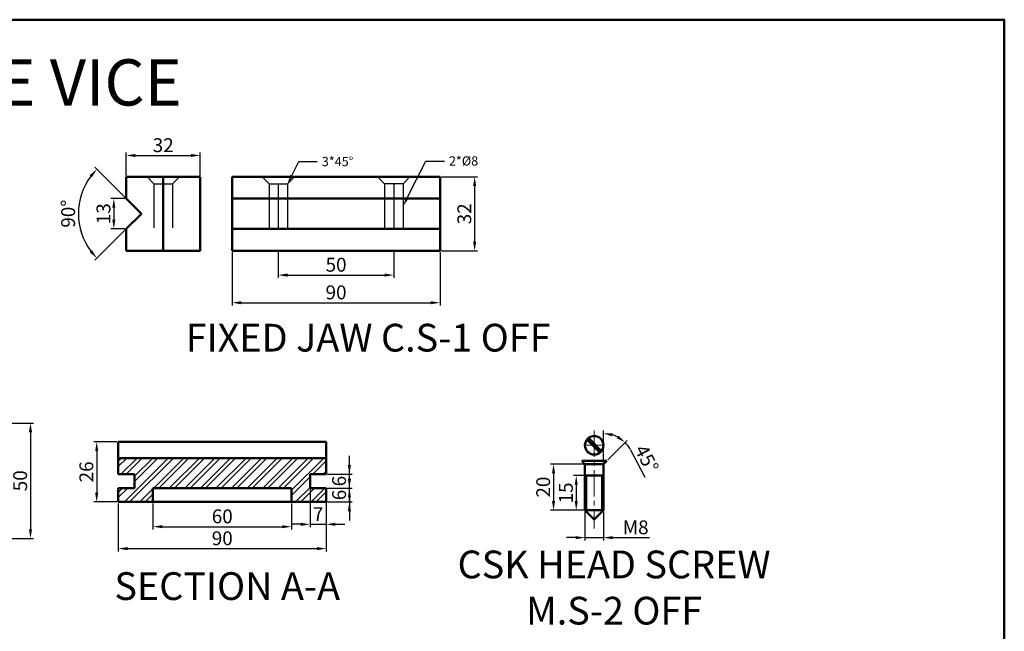
# Model space of a CAD drawing. Units: millimetres. Extents: x -1209 to -333, y 66 to 707.
# Tile 4 of 4: x -759 to -333, y 442 to 707. Entities that reach past the tile are written whole.
import ezdxf
from ezdxf import colors
from ezdxf.entities.mleader import LeaderData, LeaderLine
from ezdxf.math import Vec2, Vec3

# ---------------------------------------------------------------- set-up
doc = ezdxf.new("R2010")
doc.units = ezdxf.units.MM
doc.header["$LTSCALE"] = 1.5
doc.linetypes.add('CENTER2', pattern=[28.575, 19.05, -3.175, 3.175, -3.175])
doc.linetypes.add('DASHED', pattern=[19.05, 12.7, -6.35])
for name, color, linetype, lineweight in [('M-CNTR', 1, 'CENTER2', 18), ('M-DIMS', 2, 'Continuous', 25), ('M-HATC', 8, 'Continuous', 18), ('M-HIDN', 4, 'DASHED', 25), ('M-OUTL', 7, 'Continuous', 50), ('M-TEXT', 3, 'Continuous', 25), ('M-TTLB', 7, 'Continuous', 50)]:
    doc.layers.add(name, color=color, linetype=linetype, lineweight=lineweight)
doc.styles.get("Standard").update_dxf_attribs({"font": 'arial.ttf'})
doc.dimstyles.new('ISO-25', dxfattribs={"dimtxt": 6, "dimasz": 4, "dimexe": 1.25, "dimexo": 0.625, "dimtad": 1, "dimdec": 0, "dimtxsty": 'Standard', "dimcen": 2.5, "dimadec": 0, "dimazin": 0, "dimtfac": 1, "dimtdec": 0, "dimtmove": 0, "dimatfit": 3, "dimfxl": 1, "dimarcsym": 0})

# ---------------------------------------------------------------- blocks, each defined once
blk = doc.blocks.new('*D5')
at = {"layer": 'Defpoints', "color": 0, "transparency": 16777216}
for p in [(-788.18, 532.21), (-788.18, 482.21), (-754.08, 482.21)]:
    blk.add_point(p, dxfattribs=at)
at = {"layer": 'M-DIMS', "color": 0, "lineweight": -2, "transparency": 16777216}
for p, q in [((-787.56, 532.21), (-752.83, 532.21)), ((-754.08, 528.21), (-754.08, 486.21)), ((-787.56, 482.21), (-752.83, 482.21))]:
    blk.add_line(p, q, dxfattribs=at)
at = {"layer": 'M-DIMS', "color": 0, "transparency": 16777216}
for points in [[(-754.75, 528.21), (-753.41, 528.21), (-754.08, 532.21)], [(-754.75, 486.21), (-753.41, 486.21), (-754.08, 482.21)]]:
    blk.add_solid(points, dxfattribs=at)
at = {"layer": 'M-DIMS', "color": 0, "transparency": 16777216, "insert": (-757.77, 507.21), "char_height": 6, "attachment_point": 5, "rotation": 90}
blk.add_mtext('50', dxfattribs=at)
blk = doc.blocks.new('*D18')
at = {"layer": 'Defpoints', "color": 0, "transparency": 16777216}
for p in [(-716.06, 524.06), (-725.42, 498.06), (-716.06, 498.06)]:
    blk.add_point(p, dxfattribs=at)
at = {"layer": 'M-DIMS', "color": 0, "lineweight": -2, "transparency": 16777216}
for p, q in [((-716.69, 524.06), (-726.67, 524.06)), ((-725.42, 520.06), (-725.42, 502.06)), ((-716.69, 498.06), (-726.67, 498.06))]:
    blk.add_line(p, q, dxfattribs=at)
at = {"layer": 'M-DIMS', "color": 0, "transparency": 16777216}
for points in [[(-726.09, 520.06), (-724.76, 520.06), (-725.42, 524.06)], [(-726.09, 502.06), (-724.76, 502.06), (-725.42, 498.06)]]:
    blk.add_solid(points, dxfattribs=at)
at = {"layer": 'M-DIMS', "color": 0, "transparency": 16777216, "insert": (-729.11, 511.06), "char_height": 6, "attachment_point": 5, "rotation": 90}
blk.add_mtext('26', dxfattribs=at)
blk = doc.blocks.new('*D19')
at = {"layer": 'Defpoints', "color": 0, "transparency": 16777216}
for p in [(-716.06, 498.06), (-626.06, 498.06), (-626.06, 477.85)]:
    blk.add_point(p, dxfattribs=at)
at = {"layer": 'M-DIMS', "color": 0, "lineweight": -2, "transparency": 16777216}
for p, q in [((-716.06, 497.44), (-716.06, 476.6)), ((-626.06, 497.44), (-626.06, 476.6)), ((-712.06, 477.85), (-630.06, 477.85))]:
    blk.add_line(p, q, dxfattribs=at)
at = {"layer": 'M-DIMS', "color": 0, "transparency": 16777216}
for points in [[(-712.06, 478.52), (-712.06, 477.19), (-716.06, 477.85)], [(-630.06, 478.52), (-630.06, 477.19), (-626.06, 477.85)]]:
    blk.add_solid(points, dxfattribs=at)
at = {"layer": 'M-DIMS', "color": 0, "transparency": 16777216, "insert": (-671.06, 481.54), "char_height": 6, "attachment_point": 5}
blk.add_mtext('90', dxfattribs=at)
blk = doc.blocks.new('*D20')
at = {"layer": 'Defpoints', "color": 0, "transparency": 16777216}
for p in [(-701.06, 498.06), (-641.06, 498.06), (-641.06, 487.35)]:
    blk.add_point(p, dxfattribs=at)
at = {"layer": 'M-DIMS', "color": 0, "lineweight": -2, "transparency": 16777216}
for p, q in [((-701.06, 497.44), (-701.06, 486.1)), ((-641.06, 497.44), (-641.06, 486.1)), ((-697.06, 487.35), (-645.06, 487.35))]:
    blk.add_line(p, q, dxfattribs=at)
at = {"layer": 'M-DIMS', "color": 0, "transparency": 16777216}
for points in [[(-697.06, 488.01), (-697.06, 486.68), (-701.06, 487.35)], [(-645.06, 488.01), (-645.06, 486.68), (-641.06, 487.35)]]:
    blk.add_solid(points, dxfattribs=at)
at = {"layer": 'M-DIMS', "color": 0, "transparency": 16777216, "insert": (-671.06, 491.04), "char_height": 6, "attachment_point": 5}
blk.add_mtext('60', dxfattribs=at)
blk = doc.blocks.new('*D21')
at = {"layer": 'Defpoints', "color": 0, "transparency": 16777216}
for p in [(-633.06, 504.06), (-626.06, 504.06), (-626.06, 488.37)]:
    blk.add_point(p, dxfattribs=at)
at = {"layer": 'M-DIMS', "color": 0, "lineweight": -2, "transparency": 16777216}
for p, q in [((-633.06, 503.44), (-633.06, 487.12)), ((-626.06, 503.44), (-626.06, 487.12)), ((-637.06, 488.37), (-641.06, 488.37)), ((-633.06, 488.37), (-626.06, 488.37)), ((-622.06, 488.37), (-618.06, 488.37))]:
    blk.add_line(p, q, dxfattribs=at)
at = {"layer": 'M-DIMS', "color": 0, "transparency": 16777216}
for points in [[(-637.06, 489.04), (-637.06, 487.7), (-633.06, 488.37)], [(-622.06, 489.04), (-622.06, 487.7), (-626.06, 488.37)]]:
    blk.add_solid(points, dxfattribs=at)
at = {"layer": 'M-DIMS', "color": 0, "transparency": 16777216, "insert": (-629.56, 491.99), "char_height": 6, "attachment_point": 5}
blk.add_mtext('7', dxfattribs=at)
blk = doc.blocks.new('*D22')
at = {"layer": 'Defpoints', "color": 0, "transparency": 16777216}
for p in [(-626.06, 504.06), (-616.02, 504.06), (-626.06, 498.06)]:
    blk.add_point(p, dxfattribs=at)
at = {"layer": 'M-DIMS', "color": 0, "lineweight": -2, "transparency": 16777216}
for p, q in [((-616.02, 508.06), (-616.02, 512.06)), ((-625.44, 504.06), (-614.77, 504.06)), ((-616.02, 498.06), (-616.02, 504.06)), ((-625.44, 498.06), (-614.77, 498.06)), ((-616.02, 494.06), (-616.02, 490.06))]:
    blk.add_line(p, q, dxfattribs=at)
at = {"layer": 'M-DIMS', "color": 0, "transparency": 16777216}
for points in [[(-616.69, 508.06), (-615.35, 508.06), (-616.02, 504.06)], [(-616.69, 494.06), (-615.35, 494.06), (-616.02, 498.06)]]:
    blk.add_solid(points, dxfattribs=at)
at = {"layer": 'M-DIMS', "color": 0, "transparency": 16777216, "insert": (-619.71, 501.06), "char_height": 6, "attachment_point": 5, "rotation": 90}
blk.add_mtext('6', dxfattribs=at)
blk = doc.blocks.new('*D23')
at = {"layer": 'Defpoints', "color": 0, "transparency": 16777216}
for p in [(-626.06, 510.06), (-616.02, 510.06), (-626.06, 504.06)]:
    blk.add_point(p, dxfattribs=at)
at = {"layer": 'M-DIMS', "color": 0, "lineweight": -2, "transparency": 16777216}
for p, q in [((-616.02, 514.06), (-616.02, 518.06)), ((-625.44, 510.06), (-614.77, 510.06)), ((-616.02, 504.06), (-616.02, 510.06)), ((-625.44, 504.06), (-614.77, 504.06)), ((-616.02, 500.06), (-616.02, 496.06))]:
    blk.add_line(p, q, dxfattribs=at)
at = {"layer": 'M-DIMS', "color": 0, "transparency": 16777216}
for points in [[(-616.69, 514.06), (-615.35, 514.06), (-616.02, 510.06)], [(-616.69, 500.06), (-615.35, 500.06), (-616.02, 504.06)]]:
    blk.add_solid(points, dxfattribs=at)
at = {"layer": 'M-DIMS', "color": 0, "transparency": 16777216, "insert": (-619.71, 507.06), "char_height": 6, "attachment_point": 5, "rotation": 90}
blk.add_mtext('6', dxfattribs=at)
blk = doc.blocks.new('*D53')
at = {"layer": 'Defpoints', "color": 0, "ltscale": 0.4, "transparency": 16777216}
for p in [(-646.8, 606.73), (-596.8, 606.73), (-596.8, 596.22)]:
    blk.add_point(p, dxfattribs=at)
at = {"layer": 'M-DIMS', "color": 0, "lineweight": -2, "ltscale": 0.4, "transparency": 16777216}
for p, q in [((-646.8, 606.1), (-646.8, 594.97)), ((-596.8, 606.1), (-596.8, 594.97)), ((-642.8, 596.22), (-600.8, 596.22))]:
    blk.add_line(p, q, dxfattribs=at)
at = {"layer": 'M-DIMS', "color": 0, "ltscale": 0.4, "transparency": 16777216}
for points in [[(-642.8, 596.89), (-642.8, 595.55), (-646.8, 596.22)], [(-600.8, 596.89), (-600.8, 595.55), (-596.8, 596.22)]]:
    blk.add_solid(points, dxfattribs=at)
at = {"layer": 'M-DIMS', "color": 0, "ltscale": 0.4, "transparency": 16777216, "insert": (-621.8, 599.91), "char_height": 6, "attachment_point": 5}
blk.add_mtext('50', dxfattribs=at)
blk = doc.blocks.new('*D54')
at = {"layer": 'Defpoints', "color": 0, "ltscale": 0.4, "transparency": 16777216}
for p in [(-666.8, 606.73), (-576.8, 606.73), (-576.8, 584.26)]:
    blk.add_point(p, dxfattribs=at)
at = {"layer": 'M-DIMS', "color": 0, "lineweight": -2, "ltscale": 0.4, "transparency": 16777216}
for p, q in [((-666.8, 606.1), (-666.8, 583.01)), ((-576.8, 606.1), (-576.8, 583.01)), ((-662.8, 584.26), (-580.8, 584.26))]:
    blk.add_line(p, q, dxfattribs=at)
at = {"layer": 'M-DIMS', "color": 0, "ltscale": 0.4, "transparency": 16777216}
for points in [[(-662.8, 584.92), (-662.8, 583.59), (-666.8, 584.26)], [(-580.8, 584.92), (-580.8, 583.59), (-576.8, 584.26)]]:
    blk.add_solid(points, dxfattribs=at)
at = {"layer": 'M-DIMS', "color": 0, "ltscale": 0.4, "transparency": 16777216, "insert": (-621.8, 587.95), "char_height": 6, "attachment_point": 5}
blk.add_mtext('90', dxfattribs=at)
blk = doc.blocks.new('*D55')
at = {"layer": 'Defpoints', "color": 0, "ltscale": 0.4, "transparency": 16777216}
for p in [(-576.8, 638.73), (-576.8, 606.73), (-561.82, 606.73)]:
    blk.add_point(p, dxfattribs=at)
at = {"layer": 'M-DIMS', "color": 0, "lineweight": -2, "ltscale": 0.4, "transparency": 16777216}
for p, q in [((-576.17, 638.73), (-560.57, 638.73)), ((-561.82, 634.73), (-561.82, 610.73)), ((-576.17, 606.73), (-560.57, 606.73))]:
    blk.add_line(p, q, dxfattribs=at)
at = {"layer": 'M-DIMS', "color": 0, "ltscale": 0.4, "transparency": 16777216}
for points in [[(-562.49, 634.73), (-561.15, 634.73), (-561.82, 638.73)], [(-562.49, 610.73), (-561.15, 610.73), (-561.82, 606.73)]]:
    blk.add_solid(points, dxfattribs=at)
at = {"layer": 'M-DIMS', "color": 0, "ltscale": 0.4, "transparency": 16777216, "insert": (-565.51, 622.73), "char_height": 6, "attachment_point": 5, "rotation": 90}
blk.add_mtext('32', dxfattribs=at)
blk = doc.blocks.new('*D56')
at = {"layer": 'Defpoints', "color": 0, "ltscale": 0.4, "transparency": 16777216}
for p in [(-680.62, 647.97), (-712.62, 638.73), (-680.62, 638.73)]:
    blk.add_point(p, dxfattribs=at)
at = {"layer": 'M-DIMS', "color": 0, "lineweight": -2, "ltscale": 0.4, "transparency": 16777216}
for p, q in [((-712.62, 639.35), (-712.62, 649.22)), ((-708.62, 647.97), (-684.62, 647.97)), ((-680.62, 639.35), (-680.62, 649.22))]:
    blk.add_line(p, q, dxfattribs=at)
at = {"layer": 'M-DIMS', "color": 0, "ltscale": 0.4, "transparency": 16777216}
for points in [[(-708.62, 648.64), (-708.62, 647.31), (-712.62, 647.97)], [(-684.62, 648.64), (-684.62, 647.31), (-680.62, 647.97)]]:
    blk.add_solid(points, dxfattribs=at)
at = {"layer": 'M-DIMS', "color": 0, "ltscale": 0.4, "transparency": 16777216, "insert": (-696.62, 651.66), "char_height": 6, "attachment_point": 5}
blk.add_mtext('32', dxfattribs=at)
blk = doc.blocks.new('*D57')
at = {"layer": 'Defpoints', "color": 0, "ltscale": 0.4, "transparency": 16777216}
for p in [(-712.62, 629.33), (-718.01, 616.23), (-712.62, 616.23)]:
    blk.add_point(p, dxfattribs=at)
at = {"layer": 'M-DIMS', "color": 0, "lineweight": -2, "ltscale": 0.4, "transparency": 16777216}
for p, q in [((-713.24, 629.33), (-719.26, 629.33)), ((-718.01, 625.33), (-718.01, 620.23)), ((-713.24, 616.23), (-719.26, 616.23))]:
    blk.add_line(p, q, dxfattribs=at)
at = {"layer": 'M-DIMS', "color": 0, "ltscale": 0.4, "transparency": 16777216}
for points in [[(-718.67, 625.33), (-717.34, 625.33), (-718.01, 629.33)], [(-718.67, 620.23), (-717.34, 620.23), (-718.01, 616.23)]]:
    blk.add_solid(points, dxfattribs=at)
at = {"layer": 'M-DIMS', "color": 0, "ltscale": 0.4, "transparency": 16777216, "insert": (-721.7, 622.78), "char_height": 6, "attachment_point": 5, "rotation": 90}
blk.add_mtext('13', dxfattribs=at)
blk = doc.blocks.new('*D58')
at = {"layer": 'Defpoints', "color": 0, "ltscale": 0.4, "transparency": 16777216}
for p in [(-732.39, 629.83), (-712.62, 629.33), (-706.07, 622.78), (-706.07, 622.78), (-712.62, 616.23)]:
    blk.add_point(p, dxfattribs=at)
at = {"layer": 'M-DIMS', "color": 0, "lineweight": -2, "ltscale": 0.4, "transparency": 16777216}
for p, q in [((-713.06, 629.77), (-726.22, 642.93)), ((-713.06, 615.79), (-726.22, 602.63))]:
    blk.add_line(p, q, dxfattribs=at)
blk.add_arc((-706.07, 622.78), 27.25, 143.4187, 216.5813, dxfattribs=at)
at = {"layer": 'M-DIMS', "color": 0, "ltscale": 0.4, "transparency": 16777216}
for points in [[(-728.45, 639.45), (-727.44, 638.58), (-725.33, 642.05)], [(-727.44, 606.98), (-728.45, 606.1), (-725.33, 603.51)]]:
    blk.add_solid(points, dxfattribs=at)
at = {"layer": 'M-DIMS', "color": 0, "ltscale": 0.4, "transparency": 16777216, "insert": (-737, 622.78), "char_height": 6, "attachment_point": 5, "rotation": 90}
blk.add_mtext('90°', dxfattribs=at)
blk = doc.blocks.new('*D59')
at = {"layer": 'Defpoints', "color": 0, "ltscale": 0.4, "transparency": 16777216}
for p in [(-502.64, 527.23), (-504.65, 515.88), (-506.06, 514.46), (-506.06, 514.46), (-506.06, 494.46)]:
    blk.add_point(p, dxfattribs=at)
at = {"layer": 'M-DIMS', "color": 0, "lineweight": -2, "ltscale": 0.4, "transparency": 16777216}
for p, q in [((-506.06, 515.09), (-506.06, 528.94)), ((-504.2, 516.32), (-495.83, 524.7)), ((-494.34, 520.59), (-488.2, 508.84))]:
    blk.add_line(p, q, dxfattribs=at)
for start, end in [(62.398, 72.602), (27.602, 45)]:
    blk.add_arc((-506.06, 514.46), 13.22, start, end, dxfattribs=at)
at = {"layer": 'M-DIMS', "color": 0, "ltscale": 0.4, "transparency": 16777216}
for points in [[(-502.21, 526.42), (-502.01, 527.74), (-506.06, 527.69)], [(-499.54, 526.72), (-500.33, 525.64), (-496.71, 523.81)]]:
    blk.add_solid(points, dxfattribs=at)
at = {"layer": 'M-DIMS', "color": 0, "ltscale": 0.4, "transparency": 16777216, "insert": (-488.01, 516.42), "char_height": 6, "attachment_point": 5, "rotation": 297.602}
blk.add_mtext('45°', dxfattribs=at)
blk = doc.blocks.new('*D60')
at = {"layer": 'Defpoints', "color": 0, "ltscale": 0.4, "transparency": 16777216}
for p in [(-514.06, 514.46), (-527.66, 494.46), (-514.06, 494.46)]:
    blk.add_point(p, dxfattribs=at)
at = {"layer": 'M-DIMS', "color": 0, "lineweight": -2, "ltscale": 0.4, "transparency": 16777216}
for p, q in [((-514.69, 514.46), (-528.91, 514.46)), ((-527.66, 510.46), (-527.66, 498.46)), ((-514.69, 494.46), (-528.91, 494.46))]:
    blk.add_line(p, q, dxfattribs=at)
at = {"layer": 'M-DIMS', "color": 0, "ltscale": 0.4, "transparency": 16777216}
for points in [[(-528.33, 510.46), (-526.99, 510.46), (-527.66, 514.46)], [(-528.33, 498.46), (-526.99, 498.46), (-527.66, 494.46)]]:
    blk.add_solid(points, dxfattribs=at)
at = {"layer": 'M-DIMS', "color": 0, "ltscale": 0.4, "transparency": 16777216, "insert": (-531.35, 504.46), "char_height": 6, "attachment_point": 5, "rotation": 90}
blk.add_mtext('20', dxfattribs=at)
blk = doc.blocks.new('*D61')
at = {"layer": 'Defpoints', "color": 0, "ltscale": 0.4, "transparency": 16777216}
for p in [(-514.06, 509.46), (-517.84, 494.46), (-514.06, 494.46)]:
    blk.add_point(p, dxfattribs=at)
at = {"layer": 'M-DIMS', "color": 0, "lineweight": -2, "ltscale": 0.4, "transparency": 16777216}
for p, q in [((-514.69, 509.46), (-519.09, 509.46)), ((-517.84, 505.46), (-517.84, 498.46)), ((-514.69, 494.46), (-519.09, 494.46))]:
    blk.add_line(p, q, dxfattribs=at)
at = {"layer": 'M-DIMS', "color": 0, "ltscale": 0.4, "transparency": 16777216}
for points in [[(-518.5, 505.46), (-517.17, 505.46), (-517.84, 509.46)], [(-518.5, 498.46), (-517.17, 498.46), (-517.84, 494.46)]]:
    blk.add_solid(points, dxfattribs=at)
at = {"layer": 'M-DIMS', "color": 0, "ltscale": 0.4, "transparency": 16777216, "insert": (-521.53, 501.96), "char_height": 6, "attachment_point": 5, "rotation": 90}
blk.add_mtext('15', dxfattribs=at)
blk = doc.blocks.new('*D62')
at = {"layer": 'Defpoints', "color": 0, "ltscale": 0.4, "transparency": 16777216}
for p in [(-514.06, 494.46), (-506.06, 494.46), (-506.06, 482.61)]:
    blk.add_point(p, dxfattribs=at)
at = {"layer": 'M-DIMS', "color": 0, "lineweight": -2, "ltscale": 0.4, "transparency": 16777216}
for p, q in [((-514.06, 493.84), (-514.06, 481.36)), ((-506.06, 493.84), (-506.06, 481.36)), ((-518.06, 482.61), (-522.06, 482.61)), ((-514.06, 482.61), (-506.06, 482.61)), ((-502.06, 482.61), (-486.16, 482.61))]:
    blk.add_line(p, q, dxfattribs=at)
at = {"layer": 'M-DIMS', "color": 0, "ltscale": 0.4, "transparency": 16777216}
for points in [[(-518.06, 483.27), (-518.06, 481.94), (-514.06, 482.61)], [(-502.06, 483.27), (-502.06, 481.94), (-506.06, 482.61)]]:
    blk.add_solid(points, dxfattribs=at)
at = {"layer": 'M-DIMS', "color": 0, "ltscale": 0.4, "transparency": 16777216, "insert": (-492.11, 486.3), "char_height": 6, "attachment_point": 5}
blk.add_mtext('M8', dxfattribs=at)

msp = doc.modelspace()

# ---------------------------------------------------------------- hatches: boundary and pattern name
at = {"layer": 'M-HATC'}
h = msp.add_hatch(dxfattribs=at)
h.set_pattern_fill('ANSI32', color=256, scale=0.5)
h.set_pattern_definition([(45, (-2142.44, -526.8178), (-3.367596, 3.367596), []), (45, (-2140.195, -526.8178), (-3.367596, 3.367596), [])])
h.paths.add_polyline_path([(-641.06, 504.06), (-641.06, 498.06), (-626.06, 498.06), (-626.06, 504.06), (-633.06, 504.06), (-633.06, 510.06), (-626.06, 510.06), (-626.06, 517.06), (-638.06, 517.06), (-716.06, 517.06), (-716.06, 510.06), (-709.06, 510.06), (-709.06, 504.06), (-716.06, 504.06), (-716.06, 498.06), (-701.06, 498.06), (-701.06, 504.06)])

# ---------------------------------------------------------------- linework, layer by layer
at = {"layer": 'M-CNTR', "ltscale": 0.4}
for p, q in [((-510.06, 528.96), (-510.06, 486.51)), ((-514.06, 522.56), (-506.06, 522.56))]:
    msp.add_line(p, q, dxfattribs=at)
at = {"layer": 'M-HIDN'}
for p, q in [((-700.62, 635.73), (-703.62, 638.73)), ((-700.62, 635.73), (-700.62, 606.73)), ((-700.62, 635.73), (-692.62, 635.73)), ((-696.62, 635.73), (-696.62, 606.73)), ((-692.62, 635.73), (-689.62, 638.73)), ((-692.62, 635.73), (-692.62, 606.73)), ((-650.8, 635.73), (-653.8, 638.73)), ((-650.8, 635.73), (-650.8, 606.73)), ((-650.8, 635.73), (-642.8, 635.73)), ((-646.8, 635.73), (-646.8, 606.73)), ((-642.8, 635.73), (-639.8, 638.73)), ((-642.8, 635.73), (-642.8, 606.73)), ((-600.8, 635.73), (-603.8, 638.73)), ((-600.8, 635.73), (-600.8, 606.73)), ((-592.8, 635.73), (-600.8, 635.73)), ((-596.8, 635.73), (-596.8, 606.73)), ((-592.8, 635.73), (-589.8, 638.73)), ((-592.8, 635.73), (-592.8, 606.73))]:
    msp.add_line(p, q, dxfattribs=at)
at = {"layer": 'M-OUTL'}
for p, q in [((-712.62, 638.73), (-680.62, 638.73)), ((-712.62, 629.33), (-712.62, 638.73)), ((-700.62, 638.73), (-692.62, 638.73)), ((-680.62, 638.73), (-680.62, 606.73)), ((-576.8, 638.73), (-666.8, 638.73)), ((-666.8, 638.73), (-666.8, 606.73)), ((-592.8, 638.73), (-600.8, 638.73)), ((-576.8, 606.73), (-576.8, 638.73)), ((-666.8, 629.33), (-576.8, 629.33)), ((-712.62, 606.73), (-712.62, 616.23)), ((-666.8, 616.23), (-576.8, 616.23)), ((-680.62, 606.73), (-712.62, 606.73)), ((-666.8, 606.73), (-576.8, 606.73)), ((-716.06, 524.06), (-626.06, 524.06)), ((-716.06, 510.06), (-716.06, 524.06)), ((-626.06, 524.06), (-626.06, 510.06)), ((-638.06, 517.06), (-716.06, 517.06)), ((-626.06, 517.06), (-638.06, 517.06)), ((-709.06, 510.06), (-716.06, 510.06)), ((-709.06, 504.06), (-709.06, 510.06)), ((-626.06, 510.06), (-633.06, 510.06)), ((-633.06, 510.06), (-633.06, 504.06)), ((-716.06, 498.06), (-716.06, 504.06)), ((-709.06, 504.06), (-716.06, 504.06)), ((-641.06, 504.06), (-701.06, 504.06)), ((-701.06, 498.06), (-701.06, 504.06)), ((-641.06, 498.06), (-641.06, 504.06)), ((-626.06, 504.06), (-633.06, 504.06)), ((-626.06, 504.06), (-626.06, 498.06)), ((-626.06, 498.06), (-716.06, 498.06))]:
    msp.add_line(p, q, dxfattribs=at)
at = {"layer": 'M-OUTL', "ltscale": 0.4}
for p, q in [((-696.62, 638.73), (-696.62, 606.73)), ((-712.62, 629.33), (-706.07, 622.78)), ((-712.62, 616.23), (-706.07, 622.78)), ((-507.59, 519.38), (-513.24, 525.04)), ((-507.23, 519.74), (-512.89, 525.39)), ((-506.88, 520.09), (-512.54, 525.75)), ((-514.06, 514.46), (-515.47, 515.88)), ((-515.47, 515.88), (-504.65, 515.88)), ((-506.06, 514.46), (-504.65, 515.88)), ((-514.06, 514.46), (-506.06, 514.46)), ((-514.06, 494.46), (-514.06, 514.46)), ((-506.06, 514.46), (-506.06, 494.46)), ((-506.06, 509.46), (-514.06, 509.46)), ((-513.56, 494.46), (-513.56, 509.46)), ((-506.56, 509.46), (-506.56, 494.46)), ((-506.06, 494.46), (-514.06, 494.46)), ((-514.06, 494.46), (-510.06, 490.46)), ((-506.06, 494.46), (-510.06, 490.46))]:
    msp.add_line(p, q, dxfattribs=at)
msp.add_circle((-510.06, 522.56), 4, dxfattribs=at)
at = {"layer": 'M-TTLB', "ltscale": 0.4}
msp.add_lwpolyline([(-1209.09, 706.73), (-332.54, 706.73), (-332.54, 66.01), (-1209.09, 66.01)], close=True, dxfattribs=at)

# ---------------------------------------------------------------- texts
at = {"layer": 'M-TEXT', "ltscale": 0.4, "attachment_point": 1}
for s, width, insert, char_height in [('\\pxqc;MACHINE VICE', 213.0298, (-886.63, 689.59), 20), ('\\pxqc;FIXED JAW C.S-1 OFF', 177.8457, (-696.84, 575.13), 12), ('\\pxqc;CSK HEAD SCREW M.S-2 OFF', 177.8457, (-590.37, 477.01), 12), ('\\pxqc;SECTION A-A', 177.8457, (-757.83, 467.64), 12)]:
    msp.add_mtext_dynamic_manual_height_columns(s, width=width, gutter_width=12.5, heights=[0], dxfattribs=dict(at, insert=insert, char_height=char_height))

# ---------------------------------------------------------------- dimensions: what is measured, and where the dimension line sits
at = {"layer": 'M-DIMS', "ltscale": 0.4}
for base, p1, p2, picture, middle in [((-680.62, 647.97), (-712.62, 638.73), (-680.62, 638.73), '*D56', (-696.62, 651.66)), ((-576.8, 584.26), (-666.8, 606.73), (-576.8, 606.73), '*D54', (-621.8, 587.95)), ((-596.8, 596.22), (-646.8, 606.73), (-596.8, 606.73), '*D53', (-621.8, 599.91))]:
    dim = msp.add_linear_dim(base=base, p1=p1, p2=p2, dimstyle='ISO-25', override={"dimclrd": 0, "dimclre": 0, "dimclrt": 0}, dxfattribs=at)
    dim.commit()
    dim.dimension.update_dxf_attribs({"geometry": picture, "text_midpoint": middle})
for base, line1, line2, picture, middle in [((-732.39, 629.83), ((-712.62, 616.23), (-706.07, 622.78)), ((-712.62, 629.33), (-706.07, 622.78)), '*D58', (-737, 622.78)), ((-502.64, 527.23), ((-506.06, 514.46), (-506.06, 494.46)), ((-506.06, 514.46), (-504.65, 515.88)), '*D59', (-488.01, 516.42))]:
    dim = msp.add_angular_dim_2l(base=base, line1=line1, line2=line2, dimstyle='ISO-25', override={"dimclrd": 0, "dimclre": 0, "dimclrt": 0}, dxfattribs=at)
    dim.commit()
    dim.dimension.update_dxf_attribs({"geometry": picture, "text_midpoint": middle})
for base, p1, p2, picture, middle in [((-561.82, 606.73), (-576.8, 638.73), (-576.8, 606.73), '*D55', (-565.51, 622.73)), ((-718.01, 616.23), (-712.62, 629.33), (-712.62, 616.23), '*D57', (-721.7, 622.78)), ((-527.66, 494.46), (-514.06, 514.46), (-514.06, 494.46), '*D60', (-531.35, 504.46)), ((-517.84, 494.46), (-514.06, 509.46), (-514.06, 494.46), '*D61', (-521.53, 501.96))]:
    dim = msp.add_linear_dim(base=base, p1=p1, p2=p2, angle=90, dimstyle='ISO-25', override={"dimclrd": 0, "dimclre": 0, "dimclrt": 0}, dxfattribs=at)
    dim.commit()
    dim.dimension.update_dxf_attribs({"geometry": picture, "text_midpoint": middle})
at = {"layer": 'M-DIMS'}
for base, p1, p2, picture, middle in [((-754.08, 482.21), (-788.18, 532.21), (-788.18, 482.21), '*D5', (-757.77, 507.21)), ((-725.42, 498.06), (-716.06, 524.06), (-716.06, 498.06), '*D18', (-729.11, 511.06)), ((-616.02, 510.06), (-626.06, 504.06), (-626.06, 510.06), '*D23', (-619.71, 507.06)), ((-616.02, 504.06), (-626.06, 498.06), (-626.06, 504.06), '*D22', (-619.71, 501.06))]:
    dim = msp.add_linear_dim(base=base, p1=p1, p2=p2, angle=90, dimstyle='ISO-25', override={"dimclrd": 0, "dimclre": 0, "dimclrt": 0}, dxfattribs=at)
    dim.commit()
    dim.dimension.update_dxf_attribs({"geometry": picture, "text_midpoint": middle})
for base, p1, p2, picture, middle in [((-626.06, 488.37), (-633.06, 504.06), (-626.06, 504.06), '*D21', (-629.56, 488.37)), ((-626.06, 477.85), (-716.06, 498.06), (-626.06, 498.06), '*D19', (-671.06, 477.85)), ((-641.06, 487.35), (-701.06, 498.06), (-641.06, 498.06), '*D20', (-671.06, 487.35))]:
    dim = msp.add_linear_dim(base=base, p1=p1, p2=p2, dimstyle='ISO-25', override={"dimclrd": 0, "dimclre": 0, "dimclrt": 0}, dxfattribs=at)
    dim.commit()
    dim.dimension.update_dxf_attribs({"geometry": picture, "text_midpoint": middle, "dimtype": 160})
at = {"layer": 'M-DIMS', "ltscale": 0.4}
dim = msp.add_linear_dim(base=(-506.06, 482.61), p1=(-514.06, 494.46), p2=(-506.06, 494.46), text='M<>', dimstyle='ISO-25', override={"dimclrd": 0, "dimclre": 0, "dimclrt": 0}, dxfattribs=at)
dim.commit()
dim.dimension.update_dxf_attribs({"geometry": '*D62', "text_midpoint": (-492.11, 486.3)})

# ---------------------------------------------------------------- leaders
ml = msp.add_multileader_mtext('Standard', dxfattribs=at)
ml.set_content('2*%%C8', color=256)
ml.set_leader_properties()
ml.build(insert=Vec2(0, 0))
ctx = ml.context
ctx.base_point, ctx.plane_origin = Vec3(-574.93, 645.53), Vec3(-592.8, 626.04)
notes = []
notes.append((ctx, [(0, (1, 1, 0), (-582.93, 645.53), (1, 0), 8, [(0, [(-592.8, 626.04)], 0, [])])]))
ctx.mtext.insert, ctx.mtext.flow_direction = Vec3(-572.93, 647.61), 5
ml = msp.add_multileader_mtext('Standard', dxfattribs=at)
ml.set_content('3*45%%D', color=256)
ml.set_leader_properties()
ml.build(insert=Vec2(0, 0))
ctx = ml.context
ctx.base_point, ctx.plane_origin = Vec3(-629.96, 645.34), Vec3(-642.8, 635.73)
notes.append((ctx, [(0, (1, 1, 0), (-637.96, 645.34), (1, 0), 8, [(0, [(-642.8, 635.73)], 0, [])])]))
ctx.mtext.insert, ctx.mtext.flow_direction = Vec3(-627.96, 647.37), 5
for ctx, leaders in notes:
    for number, flags, end, landing, length, lines in leaders:
        leader = LeaderData()
        leader.index, (leader.has_last_leader_line, leader.has_dogleg_vector, leader.attachment_direction) = number, flags
        leader.last_leader_point, leader.dogleg_vector, leader.dogleg_length = Vec3(end), Vec3(landing), length
        for number, points, colour, breaks in lines:
            line = LeaderLine()
            line.index, line.vertices, line.color, line.breaks = number, Vec3.list(points), colors.encode_raw_color(colour), breaks
            leader.lines.append(line)
        ctx.leaders.append(leader)

doc.saveas('drawing.dxf')
